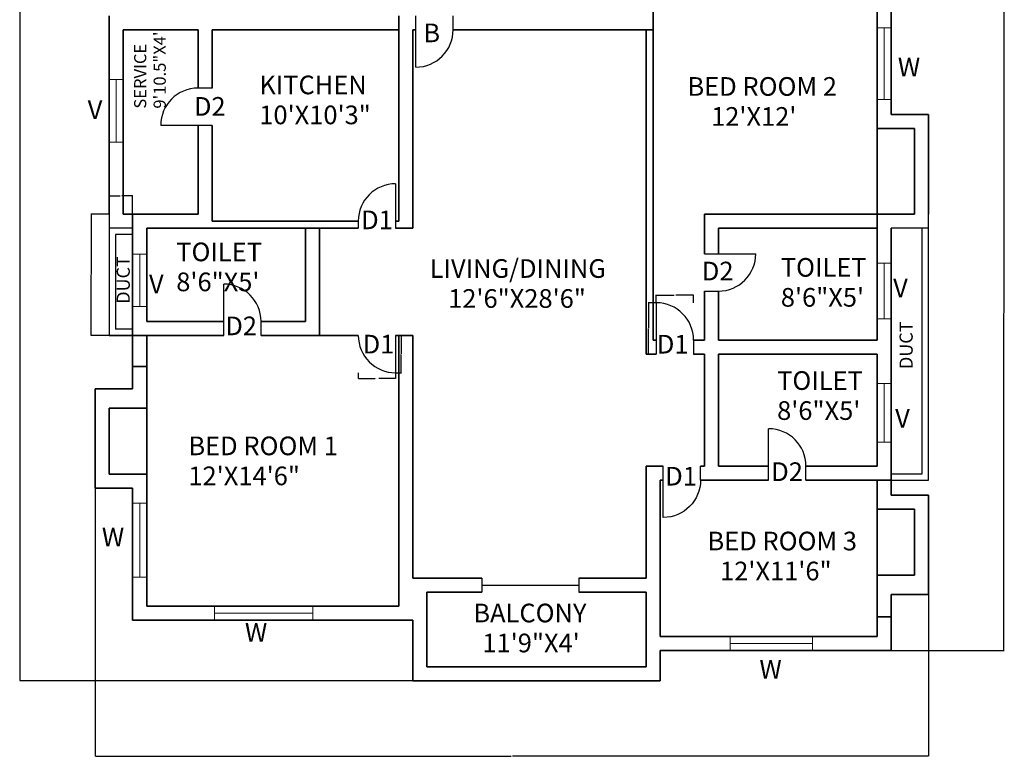
# Model space of a CAD drawing. Units: feet. Extents: x 48598101 to 48598734, y 135188346 to 135189397.
# Tile 1 of 2: x 48598101 to 48598734, y 135188346 to 135188819. Entities that reach past the tile are written whole.
import ezdxf

# ---------------------------------------------------------------- set-up
doc = ezdxf.new("R2010")
doc.units = ezdxf.units.FT
for name, color, linetype, lineweight in [('A-ANNO-DIMS', 2, 'Continuous', 18), ('A-ANNO-TEXT', 7, 'Continuous', 18), ('A-AREA-IDEN', 7, 'Continuous', 18), ('A-DOOR', 3, 'Continuous', 25), ('A-FLOR-SHFT', 7, 'Continuous', 25), ('A-GLAZ', 4, 'Continuous', 18), ('A-WALL', 7, 'Continuous', 35)]:
    doc.layers.add(name, color=color, linetype=linetype, lineweight=lineweight)
doc.styles.get("Standard").update_dxf_attribs({"font": 'arial.ttf'})
doc.dimstyles.get("Standard").update_dxf_attribs({"dimtxt": 0.18, "dimasz": 0.18, "dimexe": 0.18, "dimexo": 0.0625, "dimgap": 0.09, "dimtad": 0, "dimtih": 1, "dimtoh": 1, "dimdec": 4, "dimzin": 0, "dimdsep": 46, "dimtxsty": 'Standard', "dimcen": 0.09, "dimadec": 0, "dimazin": 0, "dimtfac": 1, "dimtdec": 4, "dimtofl": 0, "dimtmove": 0, "dimatfit": 3, "dimfxl": 1, "dimtolj": 1, "dimtzin": 0, "dimarcsym": 0})

# ---------------------------------------------------------------- blocks, each defined once
blk = doc.blocks.new('DOOR-D1-KITCHEN')
for p, q in [((24, 28.5), (24, 0)), ((0, 4.5), (0, 0))]:
    blk.add_line(p, q)
blk.add_arc((24, 4.5), 24, 90, 180)
blk = doc.blocks.new('DOOR-D1-BED-SWING')
blk.add_line((24, 24), (24, 0))
blk.add_arc((24, 24), 24, 180, 270)
blk = doc.blocks.new('DOOR-D1-BED-JAMB')
for p, q in [((0, 33), (0, 0)), ((24, 9), (24, 0))]:
    blk.add_line(p, q)
blk.add_arc((0, 9), 24, 0, 90)
blk = doc.blocks.new('DOOR-D2-SINGLE')
for p, q in [((33, 24), (24, 24)), ((33, 0), (0, 0))]:
    blk.add_line(p, q)
blk.add_arc((24, 0), 24, 90, 180)
blk = doc.blocks.new('SHAFT-VENT-NARROW')
for p, q in [((0, 78), (0, 0)), ((15, 69), (0, 69)), ((15, 65), (4, 65)), ((4, 65), (4, 4)), ((15, 4), (4, 4))]:
    blk.add_line(p, q)
blk = doc.blocks.new('*D9')
at = {"layer": 'A-ANNO-DIMS', "color": 0, "lineweight": -2, "transparency": 16777216}
for p, q in [((48598509.89, 135188637.29), (48598504.83, 135188637.29)), ((48598505.01, 135188637.11), (48598505.01, 135188620.97)), ((48598505.01, 135188604.47), (48598505.01, 135188620.61)), ((48598509.89, 135188604.29), (48598504.83, 135188604.29))]:
    blk.add_line(p, q, dxfattribs=at)
at = {"layer": 'A-ANNO-DIMS', "color": 0, "transparency": 16777216}
for points in [[(48598504.98, 135188637.11), (48598505.04, 135188637.11), (48598505.01, 135188637.29)], [(48598504.98, 135188604.47), (48598505.04, 135188604.47), (48598505.01, 135188604.29)]]:
    blk.add_solid(points, dxfattribs=at)
at = {"layer": 'Defpoints', "color": 0, "transparency": 16777216}
for p in [(48598505.01, 135188637.29), (48598509.96, 135188637.29), (48598509.96, 135188604.29)]:
    blk.add_point(p, dxfattribs=at)
at = {"layer": 'A-ANNO-DIMS', "color": 0, "transparency": 16777216, "insert": (48598505.01, 135188620.79), "char_height": 0.18, "attachment_point": 5}
blk.add_mtext('\\A1;D1 BEDROOM 33 TYP.', dxfattribs=at)
blk = doc.blocks.new('*D10')
at = {"layer": 'A-ANNO-DIMS', "color": 0, "lineweight": -2, "transparency": 16777216}
for p, q in [((48598509.96, 135188637.35), (48598509.96, 135188642.42)), ((48598510.14, 135188642.24), (48598521.43, 135188642.24)), ((48598533.78, 135188642.24), (48598522.49, 135188642.24)), ((48598533.96, 135188637.35), (48598533.96, 135188642.42))]:
    blk.add_line(p, q, dxfattribs=at)
at = {"layer": 'A-ANNO-DIMS', "color": 0, "transparency": 16777216}
for points in [[(48598510.14, 135188642.27), (48598510.14, 135188642.21), (48598509.96, 135188642.24)], [(48598533.78, 135188642.27), (48598533.78, 135188642.21), (48598533.96, 135188642.24)]]:
    blk.add_solid(points, dxfattribs=at)
at = {"layer": 'Defpoints', "color": 0, "transparency": 16777216}
for p in [(48598533.96, 135188642.24), (48598509.96, 135188637.29), (48598533.96, 135188637.29)]:
    blk.add_point(p, dxfattribs=at)
at = {"layer": 'A-ANNO-DIMS', "color": 0, "transparency": 16777216, "insert": (48598521.96, 135188642.24), "char_height": 0.18, "attachment_point": 5}
blk.add_mtext('\\A1;24 TYP.', dxfattribs=at)
blk = doc.blocks.new('*D13')
at = {"layer": 'A-ANNO-DIMS', "color": 0, "lineweight": -2, "transparency": 16777216}
for p, q in [((48598318.46, 135188592.23), (48598318.46, 135188588.51)), ((48598342.46, 135188592.23), (48598342.46, 135188588.51)), ((48598318.64, 135188588.69), (48598329.28, 135188588.69)), ((48598342.28, 135188588.69), (48598331.64, 135188588.69))]:
    blk.add_line(p, q, dxfattribs=at)
at = {"layer": 'A-ANNO-DIMS', "color": 0, "transparency": 16777216}
for points in [[(48598318.64, 135188588.72), (48598318.64, 135188588.66), (48598318.46, 135188588.69)], [(48598342.28, 135188588.72), (48598342.28, 135188588.66), (48598342.46, 135188588.69)]]:
    blk.add_solid(points, dxfattribs=at)
at = {"layer": 'Defpoints', "color": 0, "transparency": 16777216}
for p in [(48598318.46, 135188592.29), (48598342.46, 135188592.29), (48598342.46, 135188588.69)]:
    blk.add_point(p, dxfattribs=at)
at = {"layer": 'A-ANNO-DIMS', "color": 0, "transparency": 16777216, "insert": (48598330.46, 135188588.69), "char_height": 0.18, "attachment_point": 5}
blk.add_mtext('\\A1;D1 SWING 24 TYP.', dxfattribs=at)
blk = doc.blocks.new('*D14')
at = {"layer": 'A-ANNO-DIMS', "color": 0, "lineweight": -2, "transparency": 16777216}
for p, q in [((48598342.52, 135188616.29), (48598346.24, 135188616.29)), ((48598346.06, 135188616.11), (48598346.06, 135188604.47)), ((48598346.06, 135188592.47), (48598346.06, 135188604.11)), ((48598342.52, 135188592.29), (48598346.24, 135188592.29))]:
    blk.add_line(p, q, dxfattribs=at)
at = {"layer": 'A-ANNO-DIMS', "color": 0, "transparency": 16777216}
for points in [[(48598346.03, 135188616.11), (48598346.09, 135188616.11), (48598346.06, 135188616.29)], [(48598346.03, 135188592.47), (48598346.09, 135188592.47), (48598346.06, 135188592.29)]]:
    blk.add_solid(points, dxfattribs=at)
at = {"layer": 'Defpoints', "color": 0, "transparency": 16777216}
for p in [(48598342.46, 135188616.29), (48598346.06, 135188616.29), (48598342.46, 135188592.29)]:
    blk.add_point(p, dxfattribs=at)
at = {"layer": 'A-ANNO-DIMS', "color": 0, "transparency": 16777216, "insert": (48598346.06, 135188604.29), "char_height": 0.18, "attachment_point": 5}
blk.add_mtext('\\A1;24 TYP.', dxfattribs=at)
blk = doc.blocks.new('*D17')
at = {"layer": 'A-ANNO-DIMS', "color": 0, "lineweight": -2, "transparency": 16777216}
for p, q in [((48598158.39, 135188694.29), (48598146.58, 135188694.29)), ((48598146.76, 135188694.11), (48598146.76, 135188655.47)), ((48598146.76, 135188616.47), (48598146.76, 135188655.11)), ((48598158.39, 135188616.29), (48598146.58, 135188616.29))]:
    blk.add_line(p, q, dxfattribs=at)
at = {"layer": 'A-ANNO-DIMS', "color": 0, "transparency": 16777216}
for points in [[(48598146.73, 135188694.11), (48598146.79, 135188694.11), (48598146.76, 135188694.29)], [(48598146.73, 135188616.47), (48598146.79, 135188616.47), (48598146.76, 135188616.29)]]:
    blk.add_solid(points, dxfattribs=at)
at = {"layer": 'Defpoints', "color": 0, "transparency": 16777216}
for p in [(48598146.76, 135188694.29), (48598158.46, 135188694.29), (48598158.46, 135188616.29)]:
    blk.add_point(p, dxfattribs=at)
at = {"layer": 'A-ANNO-DIMS', "color": 0, "transparency": 16777216, "insert": (48598146.76, 135188655.29), "char_height": 0.18, "attachment_point": 5}
blk.add_mtext('\\A1;VENT SHAFT 78 TYP.', dxfattribs=at)
blk = doc.blocks.new('*D18')
at = {"layer": 'A-ANNO-DIMS', "color": 0, "lineweight": -2, "transparency": 16777216}
for p, q in [((48598158.46, 135188694.35), (48598158.46, 135188706.17)), ((48598158.64, 135188705.99), (48598165.44, 135188705.99)), ((48598173.28, 135188705.99), (48598166.48, 135188705.99)), ((48598173.46, 135188694.35), (48598173.46, 135188706.17))]:
    blk.add_line(p, q, dxfattribs=at)
at = {"layer": 'A-ANNO-DIMS', "color": 0, "transparency": 16777216}
for points in [[(48598158.64, 135188706.02), (48598158.64, 135188705.96), (48598158.46, 135188705.99)], [(48598173.28, 135188706.02), (48598173.28, 135188705.96), (48598173.46, 135188705.99)]]:
    blk.add_solid(points, dxfattribs=at)
at = {"layer": 'Defpoints', "color": 0, "transparency": 16777216}
for p in [(48598173.46, 135188705.99), (48598158.46, 135188694.29), (48598173.46, 135188694.29)]:
    blk.add_point(p, dxfattribs=at)
at = {"layer": 'A-ANNO-DIMS', "color": 0, "transparency": 16777216, "insert": (48598165.96, 135188705.99), "char_height": 0.18, "attachment_point": 5}
blk.add_mtext('\\A1;15 TYP.', dxfattribs=at)
blk = doc.blocks.new('*D19')
at = {"layer": 'A-ANNO-DIMS', "color": 0, "lineweight": -2, "transparency": 16777216}
for p, q in [((48598503.39, 135189348.29), (48598100.88, 135189348.29)), ((48598101.06, 135189348.11), (48598101.06, 135188871.47)), ((48598101.06, 135188394.47), (48598101.06, 135188871.11)), ((48598353.39, 135188394.29), (48598100.88, 135188394.29))]:
    blk.add_line(p, q, dxfattribs=at)
at = {"layer": 'A-ANNO-DIMS', "color": 0, "transparency": 16777216}
for points in [[(48598101.03, 135189348.11), (48598101.09, 135189348.11), (48598101.06, 135189348.29)], [(48598101.03, 135188394.47), (48598101.09, 135188394.47), (48598101.06, 135188394.29)]]:
    blk.add_solid(points, dxfattribs=at)
at = {"layer": 'Defpoints', "color": 0, "transparency": 16777216}
for p in [(48598503.46, 135189348.29), (48598101.06, 135188394.29), (48598353.46, 135188394.29)]:
    blk.add_point(p, dxfattribs=at)
at = {"layer": 'A-ANNO-DIMS', "color": 0, "transparency": 16777216, "insert": (48598101.06, 135188871.29), "char_height": 0.18, "attachment_point": 5}
blk.add_mtext('\\A1;954', dxfattribs=at)
blk = doc.blocks.new('*D20')
at = {"layer": 'A-ANNO-DIMS', "color": 0, "lineweight": -2, "transparency": 16777216}
for p, q in [((48598149.46, 135188518), (48598149.46, 135188345.71)), ((48598684.96, 135188449.7), (48598684.96, 135188345.71)), ((48598149.64, 135188345.89), (48598416.81, 135188345.89)), ((48598684.78, 135188345.89), (48598417.6, 135188345.89))]:
    blk.add_line(p, q, dxfattribs=at)
at = {"layer": 'A-ANNO-DIMS', "color": 0, "transparency": 16777216}
for points in [[(48598149.64, 135188345.92), (48598149.64, 135188345.86), (48598149.46, 135188345.89)], [(48598684.78, 135188345.92), (48598684.78, 135188345.86), (48598684.96, 135188345.89)]]:
    blk.add_solid(points, dxfattribs=at)
at = {"layer": 'Defpoints', "color": 0, "transparency": 16777216}
for p in [(48598149.46, 135188518.07), (48598684.96, 135188449.77), (48598684.96, 135188345.89)]:
    blk.add_point(p, dxfattribs=at)
at = {"layer": 'A-ANNO-DIMS', "color": 0, "transparency": 16777216, "insert": (48598417.21, 135188345.89), "char_height": 0.18, "attachment_point": 5}
blk.add_mtext('\\A1;535.5', dxfattribs=at)
blk = doc.blocks.new('*D25')
at = {"layer": 'A-ANNO-DIMS', "color": 0, "lineweight": -2, "transparency": 16777216}
for p, q in [((48598652.02, 135188847.29), (48598733.54, 135188847.29)), ((48598733.36, 135188847.11), (48598733.36, 135188630.72)), ((48598733.36, 135188413.97), (48598733.36, 135188630.36)), ((48598661.02, 135188413.79), (48598733.54, 135188413.79))]:
    blk.add_line(p, q, dxfattribs=at)
at = {"layer": 'A-ANNO-DIMS', "color": 0, "transparency": 16777216}
for points in [[(48598733.33, 135188847.11), (48598733.39, 135188847.11), (48598733.36, 135188847.29)], [(48598733.33, 135188413.97), (48598733.39, 135188413.97), (48598733.36, 135188413.79)]]:
    blk.add_solid(points, dxfattribs=at)
at = {"layer": 'Defpoints', "color": 0, "transparency": 16777216}
for p in [(48598651.96, 135188847.29), (48598660.96, 135188413.79), (48598733.36, 135188413.79)]:
    blk.add_point(p, dxfattribs=at)
at = {"layer": 'A-ANNO-DIMS', "color": 0, "transparency": 16777216, "insert": (48598733.36, 135188630.54), "char_height": 0.18, "attachment_point": 5}
blk.add_mtext('\\A1;433.5', dxfattribs=at)

msp = doc.modelspace()

# ---------------------------------------------------------------- linework, layer by layer
at = {"layer": 'A-DOOR'}
for p, q in [((48598355.46, 135188802.29), (48598355.46, 135188821.79)), ((48598379.46, 135188812.79), (48598379.46, 135188821.79)), ((48598355.46, 135188788.79), (48598355.46, 135188802.29)), ((48598509.96, 135188637.29), (48598509.96, 135188637.29)), ((48598397.79, 135188460.29), (48598397.79, 135188451.29)), ((48598460.24, 135188460.29), (48598460.24, 135188451.29)), ((48598397.79, 135188455.79), (48598460.24, 135188455.79))]:
    msp.add_line(p, q, dxfattribs=at)
msp.add_arc((48598355.46, 135188812.79), 24, 270, 360, dxfattribs=at)
at = {"layer": 'A-FLOR-SHFT'}
for p, q in [((48598684.96, 135188693.65), (48598684.96, 135188694.29)), ((48598684.96, 135188685.29), (48598660.96, 135188685.29))]:
    msp.add_line(p, q, dxfattribs=at)
for points in [[(48598651.96, 135188523.29), (48598684.96, 135188523.29), (48598684.96, 135188693.65)], [(48598660.96, 135188527.29), (48598680.96, 135188527.29), (48598680.96, 135188685.29)]]:
    msp.add_lwpolyline(points, dxfattribs=at)
at = {"layer": 'A-GLAZ'}
for p, q in [((48598651.96, 135188814.04), (48598660.96, 135188814.04)), ((48598656.46, 135188814.04), (48598656.46, 135188767.92)), ((48598158.46, 135188780.93), (48598167.46, 135188780.93)), ((48598162.96, 135188780.93), (48598162.96, 135188740.63)), ((48598651.96, 135188767.92), (48598660.96, 135188767.92)), ((48598158.46, 135188740.63), (48598167.46, 135188740.63)), ((48598173.46, 135188668.46), (48598182.46, 135188668.46)), ((48598177.96, 135188668.46), (48598177.96, 135188634.8)), ((48598651.96, 135188662.85), (48598660.96, 135188662.85)), ((48598656.46, 135188662.85), (48598656.46, 135188627.06)), ((48598173.46, 135188634.8), (48598182.46, 135188634.8)), ((48598651.96, 135188627.06), (48598660.96, 135188627.06)), ((48598651.96, 135188585.47), (48598660.96, 135188585.47)), ((48598656.46, 135188585.47), (48598656.46, 135188547.7)), ((48598651.96, 135188547.7), (48598660.96, 135188547.7)), ((48598182.46, 135188508.42), (48598173.46, 135188508.42)), ((48598177.96, 135188508.42), (48598177.96, 135188460.78)), ((48598173.46, 135188460.78), (48598182.46, 135188460.78)), ((48598226.07, 135188442.29), (48598226.07, 135188433.29)), ((48598289.26, 135188442.29), (48598289.26, 135188433.29)), ((48598226.07, 135188437.79), (48598289.26, 135188437.79)), ((48598557.44, 135188422.79), (48598557.44, 135188413.79)), ((48598610.31, 135188422.79), (48598610.31, 135188413.79)), ((48598557.44, 135188418.29), (48598610.31, 135188418.29))]:
    msp.add_line(p, q, dxfattribs=at)
at = {"layer": 'A-WALL'}
for p, q in [((48598507.96, 135188613.29), (48598507.96, 135188838.29)), ((48598651.96, 135188613.29), (48598651.96, 135188838.29)), ((48598660.96, 135188758.27), (48598660.96, 135188838.29)), ((48598158.46, 135188694.29), (48598158.46, 135188821.79)), ((48598344.46, 135188803.79), (48598344.46, 135188821.79)), ((48598167.46, 135188812.79), (48598215.46, 135188812.79)), ((48598167.46, 135188694.29), (48598167.46, 135188812.79)), ((48598215.46, 135188812.79), (48598215.46, 135188775.29)), ((48598224.46, 135188812.79), (48598224.46, 135188775.29)), ((48598224.46, 135188812.79), (48598344.46, 135188812.79)), ((48598344.46, 135188812.79), (48598344.46, 135188689.79)), ((48598353.46, 135188802.29), (48598353.46, 135188812.79)), ((48598355.46, 135188812.79), (48598353.46, 135188812.79)), ((48598355.46, 135188812.79), (48598353.46, 135188812.79)), ((48598422.46, 135188812.79), (48598379.46, 135188812.79)), ((48598503.46, 135188812.79), (48598379.46, 135188812.79)), ((48598507.96, 135188812.79), (48598422.46, 135188812.79)), ((48598503.46, 135188812.79), (48598503.46, 135188638.79)), ((48598503.46, 135188604.29), (48598503.46, 135188812.79)), ((48598353.46, 135188685.29), (48598353.46, 135188802.29)), ((48598684.96, 135188758.27), (48598660.96, 135188758.27)), ((48598684.96, 135188694.29), (48598684.96, 135188758.27)), ((48598215.46, 135188751.29), (48598215.46, 135188694.29)), ((48598224.46, 135188751.29), (48598224.46, 135188689.79)), ((48598675.96, 135188749.27), (48598651.96, 135188749.27)), ((48598675.96, 135188694.29), (48598675.96, 135188749.27)), ((48598215.46, 135188694.29), (48598167.46, 135188694.29)), ((48598173.46, 135188625.29), (48598173.46, 135188694.29)), ((48598540.96, 135188694.29), (48598540.96, 135188668.79)), ((48598675.96, 135188694.29), (48598540.96, 135188694.29)), ((48598318.46, 135188689.79), (48598224.46, 135188689.79)), ((48598344.46, 135188689.79), (48598342.46, 135188689.79)), ((48598182.46, 135188625.29), (48598182.46, 135188685.29)), ((48598318.46, 135188685.29), (48598182.46, 135188685.29)), ((48598284.46, 135188685.29), (48598284.46, 135188625.29)), ((48598293.46, 135188685.29), (48598293.46, 135188616.29)), ((48598353.46, 135188685.29), (48598342.46, 135188685.29)), ((48598540.96, 135188685.29), (48598540.96, 135188668.79)), ((48598555.96, 135188685.29), (48598549.96, 135188685.29)), ((48598549.96, 135188685.29), (48598549.96, 135188668.79)), ((48598651.96, 135188685.29), (48598555.96, 135188685.29)), ((48598660.96, 135188613.29), (48598660.96, 135188685.29)), ((48598660.96, 135188513.58), (48598660.96, 135188685.29)), ((48598540.96, 135188644.79), (48598540.96, 135188613.29)), ((48598540.96, 135188644.79), (48598540.96, 135188613.29)), ((48598549.96, 135188644.79), (48598549.96, 135188613.29)), ((48598173.46, 135188625.29), (48598173.46, 135188581.88)), ((48598231.96, 135188625.29), (48598182.46, 135188625.29)), ((48598284.46, 135188625.29), (48598255.96, 135188625.29)), ((48598231.96, 135188616.29), (48598158.46, 135188616.29)), ((48598182.46, 135188616.29), (48598182.46, 135188442.29)), ((48598318.46, 135188616.29), (48598255.96, 135188616.29)), ((48598353.46, 135188616.29), (48598342.46, 135188616.29)), ((48598344.46, 135188616.29), (48598344.46, 135188442.29)), ((48598344.46, 135188616.29), (48598344.46, 135188442.29)), ((48598353.46, 135188460.29), (48598353.46, 135188616.29)), ((48598509.96, 135188613.29), (48598507.96, 135188613.29)), ((48598540.96, 135188613.29), (48598533.96, 135188613.29)), ((48598651.96, 135188613.29), (48598549.96, 135188613.29)), ((48598509.96, 135188604.29), (48598503.46, 135188604.29)), ((48598540.96, 135188604.29), (48598533.96, 135188604.29)), ((48598540.96, 135188604.29), (48598540.96, 135188532.29)), ((48598651.96, 135188604.29), (48598549.96, 135188604.29)), ((48598549.96, 135188604.29), (48598549.96, 135188532.29)), ((48598549.96, 135188604.29), (48598549.96, 135188589.29)), ((48598651.96, 135188532.29), (48598651.96, 135188604.29)), ((48598660.96, 135188532.29), (48598660.96, 135188604.29)), ((48598182.46, 135188596.29), (48598173.46, 135188596.29)), ((48598353.46, 135188460.29), (48598353.46, 135188589.29)), ((48598149.46, 135188582.05), (48598149.46, 135188518.07)), ((48598173.46, 135188581.88), (48598149.46, 135188581.88)), ((48598158.46, 135188569.45), (48598158.46, 135188527.07)), ((48598182.46, 135188569.45), (48598158.46, 135188569.45)), ((48598503.46, 135188460.29), (48598503.46, 135188532.29)), ((48598503.46, 135188532.29), (48598503.46, 135188460.29)), ((48598514.46, 135188532.29), (48598503.46, 135188532.29)), ((48598540.96, 135188532.29), (48598538.46, 135188532.29)), ((48598582.21, 135188532.29), (48598549.96, 135188532.29)), ((48598651.96, 135188532.29), (48598606.21, 135188532.29)), ((48598158.46, 135188527.07), (48598182.46, 135188527.07)), ((48598512.46, 135188442.29), (48598512.46, 135188523.29)), ((48598514.46, 135188523.29), (48598512.46, 135188523.29)), ((48598582.21, 135188523.29), (48598538.46, 135188523.29)), ((48598651.96, 135188523.29), (48598606.21, 135188523.29)), ((48598651.96, 135188422.79), (48598651.96, 135188523.29)), ((48598651.96, 135188523.23), (48598660.96, 135188523.23)), ((48598149.46, 135188518.07), (48598173.46, 135188518.07)), ((48598173.46, 135188518.07), (48598173.46, 135188433.29)), ((48598684.96, 135188513.58), (48598660.96, 135188513.58)), ((48598684.96, 135188449.6), (48598684.96, 135188513.58)), ((48598675.96, 135188504.58), (48598651.96, 135188504.58)), ((48598675.96, 135188462.2), (48598675.96, 135188504.58)), ((48598397.79, 135188460.29), (48598353.46, 135188460.29)), ((48598503.46, 135188460.29), (48598460.24, 135188460.29)), ((48598651.96, 135188462.2), (48598675.96, 135188462.2)), ((48598362.46, 135188403.29), (48598362.46, 135188451.29)), ((48598397.79, 135188451.29), (48598362.46, 135188451.29)), ((48598503.46, 135188451.29), (48598460.24, 135188451.29)), ((48598503.46, 135188451.29), (48598503.46, 135188403.29)), ((48598512.46, 135188451.29), (48598512.46, 135188422.79)), ((48598660.96, 135188413.79), (48598660.96, 135188449.77)), ((48598660.96, 135188449.77), (48598684.96, 135188449.77)), ((48598182.46, 135188442.29), (48598344.46, 135188442.29)), ((48598353.46, 135188433.29), (48598173.46, 135188433.29)), ((48598353.46, 135188394.29), (48598353.46, 135188433.29)), ((48598651.96, 135188435.35), (48598660.96, 135188435.35)), ((48598512.46, 135188422.79), (48598651.96, 135188422.79)), ((48598512.46, 135188413.79), (48598660.96, 135188413.79)), ((48598512.46, 135188413.79), (48598512.46, 135188394.29)), ((48598503.46, 135188403.29), (48598362.46, 135188403.29)), ((48598512.46, 135188394.29), (48598353.46, 135188394.29))]:
    msp.add_line(p, q, dxfattribs=at)

# ---------------------------------------------------------------- block references
at = {"layer": 'A-DOOR'}
for name, p in [('DOOR-D2-SINGLE', (48598191.46, 135188751.29)), ('DOOR-D1-KITCHEN', (48598318.46, 135188685.29)), ('DOOR-D1-BED-JAMB', (48598509.96, 135188604.29)), ('DOOR-D1-BED-SWING', (48598318.46, 135188592.29))]:
    msp.add_blockref(name, p, dxfattribs=at)
for p, rotation in [((48598573.96, 135188668.79), 180), ((48598231.96, 135188649.29), 270.0000001790853), ((48598582.21, 135188556.29), 270.0000001790853)]:
    msp.add_blockref('DOOR-D2-SINGLE', p, dxfattribs=dict(at, rotation=rotation))
at = {"layer": 'A-DOOR', "extrusion": (0, 0, -1), "zscale": -1, "rotation": 180}
msp.add_blockref('DOOR-D1-BED-JAMB', (-48598514.46, 135188532.29), dxfattribs=at)
at = {"layer": 'A-FLOR-SHFT'}
msp.add_blockref('SHAFT-VENT-NARROW', (48598158.46, 135188616.29), dxfattribs=at)

# ---------------------------------------------------------------- texts
at = {"layer": 'A-ANNO-DIMS'}
msp.add_text('9\'10.5"X4\'', height=7.81, rotation=90, dxfattribs=at).set_placement((48598194.74, 135188762.1))
for s, p in [('10\'X10\'3"', (48598254.85, 135188752.07)), ("12'X12'", (48598545.22, 135188751.08)), ('8\'6"X5\'', (48598201.48, 135188644.72)), ('12\'6"X28\'6"', (48598376.23, 135188634.04)), ('8\'6"X5\'', (48598590.03, 135188634.78)), ('8\'6"X5\'', (48598587.65, 135188562)), ('12\'X14\'6"', (48598209.29, 135188520.01)), ('12\'X11\'6"', (48598550.99, 135188458.83)), ('11\'9"X4\'', (48598398.24, 135188412.56))]:
    msp.add_text(s, height=12, dxfattribs=at).set_placement(p)
at = {"layer": 'A-ANNO-TEXT'}
for s, p in [('W', (48598665.23, 135188782.8)), ('D2', (48598212.84, 135188757.54)), ('V', (48598144.55, 135188755.42)), ('D1', (48598320.33, 135188684.6)), ('D2', (48598539.28, 135188651.67)), ('V', (48598183.95, 135188643.42)), ('V', (48598662.22, 135188640.86)), ('D2', (48598233.01, 135188616.43)), ('D1', (48598321.28, 135188604.69)), ('D1', (48598510.37, 135188604.67)), ('V', (48598663.53, 135188557.04)), ('D2', (48598583.87, 135188522.69)), ('D1', (48598515.74, 135188519.81)), ('W', (48598153.66, 135188480.65)), ('W', (48598245.59, 135188419.41)), ('W', (48598576.26, 135188395.7))]:
    msp.add_text(s, height=12, dxfattribs=at).set_placement(p)
at = {"layer": 'A-AREA-IDEN'}
for s, p in [('B', (48598360.3, 135188804.79)), ('KITCHEN', (48598254.85, 135188771.34)), ('BED ROOM 2', (48598530.04, 135188770.36)), ('TOILET', (48598201.48, 135188664)), ('LIVING/DINING', (48598364.35, 135188653.32)), ('TOILET', (48598590.03, 135188654.05)), ('TOILET', (48598587.65, 135188581.28)), ('BED ROOM 1', (48598209.29, 135188539.28)), ('BED ROOM 3', (48598542.91, 135188478.11)), ('BALCONY', (48598392.41, 135188431.84))]:
    msp.add_text(s, height=12, dxfattribs=at).set_placement(p)
for s, height, p in [('SERVICE', 7.81, (48598182.2, 135188762.1)), ('DUCT', 8.447, (48598171.63, 135188636.68)), ('DUCT', 8.447, (48598674.78, 135188594.71))]:
    msp.add_text(s, height=height, rotation=90, dxfattribs=at).set_placement(p)

# ---------------------------------------------------------------- dimensions: what is measured, and where the dimension line sits
at = {"layer": 'A-ANNO-DIMS'}
for base, p1, p2, override, picture, middle in [((48598101.06, 135188394.29), (48598503.46, 135189348.29), (48598353.46, 135188394.29), {"dimdec": 0, "dimlfac": 1, "dimrnd": 0, "dimzin": 0, "dimdsep": 46, "dimlunit": 2}, '*D19', (48598101.06, 135188871.29)), ((48598733.36, 135188413.79), (48598651.96, 135188847.29), (48598660.96, 135188413.79), {"dimdec": 1, "dimlfac": 1, "dimrnd": 0, "dimzin": 0, "dimdsep": 46, "dimlunit": 2}, '*D25', (48598733.36, 135188630.54))]:
    dim = msp.add_linear_dim(base=base, p1=p1, p2=p2, angle=90, dimstyle='Standard', override=override, dxfattribs=at)
    dim.commit()
    dim.dimension.update_dxf_attribs({"geometry": picture, "text_midpoint": middle})
for base, p1, p2, text, picture, middle in [((48598173.46, 135188705.99), (48598158.46, 135188694.29), (48598173.46, 135188694.29), '<> TYP.', '*D18', (48598165.96, 135188705.99)), ((48598533.96, 135188642.24), (48598509.96, 135188637.29), (48598533.96, 135188637.29), '<> TYP.', '*D10', (48598521.96, 135188642.24)), ((48598342.46, 135188588.69), (48598318.46, 135188592.29), (48598342.46, 135188592.29), 'D1 SWING <> TYP.', '*D13', (48598330.46, 135188588.69))]:
    dim = msp.add_linear_dim(base=base, p1=p1, p2=p2, text=text, dimstyle='Standard', override={"dimdec": 0, "dimlfac": 1, "dimrnd": 0, "dimzin": 0, "dimdsep": 46, "dimlunit": 2}, dxfattribs=at)
    dim.commit()
    dim.dimension.update_dxf_attribs({"geometry": picture, "text_midpoint": middle})
for base, p1, p2, text, picture, middle in [((48598146.76, 135188694.29), (48598158.46, 135188616.29), (48598158.46, 135188694.29), 'VENT SHAFT <> TYP.', '*D17', (48598146.76, 135188655.29)), ((48598505.01, 135188637.29), (48598509.96, 135188604.29), (48598509.96, 135188637.29), 'D1 BEDROOM <> TYP.', '*D9', (48598505.01, 135188620.79)), ((48598346.06, 135188616.29), (48598342.46, 135188592.29), (48598342.46, 135188616.29), '<> TYP.', '*D14', (48598346.06, 135188604.29))]:
    dim = msp.add_linear_dim(base=base, p1=p1, p2=p2, angle=90, text=text, dimstyle='Standard', override={"dimdec": 0, "dimlfac": 1, "dimrnd": 0, "dimzin": 0, "dimdsep": 46, "dimlunit": 2}, dxfattribs=at)
    dim.commit()
    dim.dimension.update_dxf_attribs({"geometry": picture, "text_midpoint": middle})
dim = msp.add_linear_dim(base=(48598684.96, 135188345.89), p1=(48598149.46, 135188518.07), p2=(48598684.96, 135188449.77), dimstyle='Standard', override={"dimdec": 1, "dimlfac": 1, "dimrnd": 0, "dimzin": 0, "dimdsep": 46, "dimlunit": 2}, dxfattribs=at)
dim.commit()
dim.dimension.update_dxf_attribs({"geometry": '*D20', "text_midpoint": (48598417.21, 135188345.89)})

doc.saveas('drawing.dxf')
